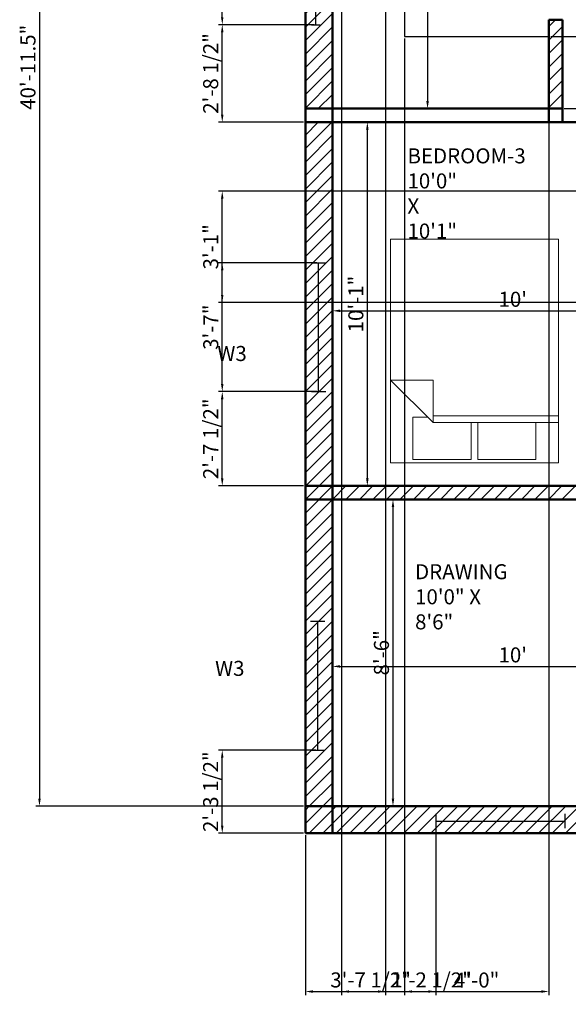
# Model space of a CAD drawing. Units: millimetres. Extents: x 2600 to 3013, y 1440 to 2066.
# Tile 1 of 4: x 2600 to 2782, y 1440 to 1768. Entities that reach past the tile are written whole.
import ezdxf

# ---------------------------------------------------------------- set-up
doc = ezdxf.new("R2010")
doc.units = ezdxf.units.MM
for name, color, linetype, lineweight in [('A-AREA-IDEN', 130, 'Continuous', 25), ('A-FLOR-CASE', 8, 'Continuous', 25), ('A-WALL-PATT', 90, 'Continuous', 13), ('dimensions', 50, 'Continuous', 18), ('furniture', 160, 'Continuous', 18), ('text', 130, 'Continuous', 18), ('walls', 90, 'Continuous', 50), ('windows', 30, 'Continuous', 25)]:
    doc.layers.add(name, color=color, linetype=linetype, lineweight=lineweight)
doc.styles.get("Standard").update_dxf_attribs({"font": 'arial.ttf'})
doc.dimstyles.new('ISO-25', dxfattribs={"dimtxt": 5, "dimasz": 2.5, "dimexe": 1.25, "dimexo": 0.625, "dimtad": 1, "dimdec": 1, "dimlunit": 3, "dimtxsty": 'Standard', "dimcen": 2.5, "dimadec": 0, "dimazin": 0, "dimtfac": 1, "dimtdec": 1, "dimtmove": 0, "dimatfit": 3, "dimfxl": 1, "dimarcsym": 0})

# ---------------------------------------------------------------- blocks, each defined once
blk = doc.blocks.new('*U4')
for p, q in [((0, 4), (0, 0)), ((0, 2), (36, 2)), ((36, 4), (36, 0))]:
    blk.add_line(p, q)
blk = doc.blocks.new('*U5')
for p, q in [((0, 4), (0, 0)), ((36, 4), (36, 0)), ((0, 2), (36, 2))]:
    blk.add_line(p, q)
blk = doc.blocks.new('Bed - Queen')
for p, q in [((0, -80.00003), (0, 0)), ((0, 0), (59.99999, 0)), ((59.99999, 0), (59.99999, -80.00003)), ((7.99999, -1.2), (28.79998, -1.2)), ((7.99999, -14.4), (7.99999, -1.2)), ((28.79998, -1.2), (28.79998, -14.4)), ((31.19999, -1.2), (51.99999, -1.2)), ((31.19999, -14.4), (31.19999, -1.2)), ((51.99999, -1.2), (51.99999, -16.4)), ((0, -14.4), (44.8, -14.4)), ((44.8, -16.8), (0, -16.8)), ((59.99999, -29.6), (44.8, -14.4)), ((44.8, -14.4), (44.8, -29.6)), ((51.99999, -16.4), (46.79936, -16.4)), ((44.8, -29.6), (59.99999, -29.6)), ((59.99999, -80.00003), (0, -80.00003))]:
    blk.add_line(p, q)
blk = doc.blocks.new('*D14')
at = {"layer": 'Defpoints', "color": 0, "transparency": 16777216}
for p in [(2735.41, 1834.18), (2735.41, 1738.18), (2735.41, 1738.18)]:
    blk.add_point(p, dxfattribs=at)
at = {"layer": 'dimensions', "color": 0, "lineweight": -2, "transparency": 16777216}
for p, q in [((2736.04, 1834.18), (2736.66, 1834.18)), ((2735.41, 1831.68), (2735.41, 1740.68)), ((2736.04, 1738.18), (2736.66, 1738.18))]:
    blk.add_line(p, q, dxfattribs=at)
at = {"layer": 'dimensions', "color": 0, "transparency": 16777216}
for points in [[(2735, 1831.68), (2735.83, 1831.68), (2735.41, 1834.18)], [(2735, 1740.68), (2735.83, 1740.68), (2735.41, 1738.18)]]:
    blk.add_solid(points, dxfattribs=at)
at = {"layer": 'dimensions', "color": 0, "transparency": 16777216, "insert": (2732.24, 1786.18), "char_height": 5, "attachment_point": 5, "rotation": 90}
blk.add_mtext("8'", dxfattribs=at)
blk = doc.blocks.new('*D18')
at = {"layer": 'Defpoints', "color": 0, "transparency": 16777216}
for p in [(2823.76, 1552.66), (2703.76, 1535.62), (2823.76, 1535.62)]:
    blk.add_point(p, dxfattribs=at)
at = {"layer": 'dimensions', "color": 0, "lineweight": -2, "transparency": 16777216}
for p, q in [((2703.76, 1536.24), (2703.76, 1553.91)), ((2706.26, 1552.66), (2821.26, 1552.66)), ((2823.76, 1536.24), (2823.76, 1553.91))]:
    blk.add_line(p, q, dxfattribs=at)
at = {"layer": 'dimensions', "color": 0, "transparency": 16777216}
for points in [[(2706.26, 1553.08), (2706.26, 1552.24), (2703.76, 1552.66)], [(2821.26, 1553.08), (2821.26, 1552.24), (2823.76, 1552.66)]]:
    blk.add_solid(points, dxfattribs=at)
at = {"layer": 'dimensions', "color": 0, "transparency": 16777216, "insert": (2763.76, 1555.84), "char_height": 5, "attachment_point": 5}
blk.add_mtext("10'", dxfattribs=at)
blk = doc.blocks.new('*D19')
at = {"layer": 'Defpoints', "color": 0, "transparency": 16777216}
for p in [(2710.05, 1608.18), (2710.05, 1506.18), (2723.9, 1506.18)]:
    blk.add_point(p, dxfattribs=at)
at = {"layer": 'dimensions', "color": 0, "lineweight": -2, "transparency": 16777216}
for p, q in [((2710.67, 1608.18), (2725.15, 1608.18)), ((2723.9, 1605.68), (2723.9, 1508.68)), ((2710.67, 1506.18), (2725.15, 1506.18))]:
    blk.add_line(p, q, dxfattribs=at)
at = {"layer": 'dimensions', "color": 0, "transparency": 16777216}
for points in [[(2723.49, 1605.68), (2724.32, 1605.68), (2723.9, 1608.18)], [(2723.49, 1508.68), (2724.32, 1508.68), (2723.9, 1506.18)]]:
    blk.add_solid(points, dxfattribs=at)
at = {"layer": 'dimensions', "color": 0, "transparency": 16777216, "insert": (2720.72, 1557.18), "char_height": 5, "attachment_point": 5, "rotation": 90}
blk.add_mtext('8\'-6"', dxfattribs=at)
blk = doc.blocks.new('*D22')
at = {"layer": 'Defpoints', "color": 0, "transparency": 16777216}
for p in [(2703.76, 1677.24), (2823.76, 1677.24), (2823.76, 1670.93)]:
    blk.add_point(p, dxfattribs=at)
at = {"layer": 'dimensions', "color": 0, "lineweight": -2, "transparency": 16777216}
for p, q in [((2703.76, 1676.61), (2703.76, 1669.68)), ((2823.76, 1676.61), (2823.76, 1669.68)), ((2706.26, 1670.93), (2821.26, 1670.93))]:
    blk.add_line(p, q, dxfattribs=at)
at = {"layer": 'dimensions', "color": 0, "transparency": 16777216}
for points in [[(2706.26, 1671.35), (2706.26, 1670.51), (2703.76, 1670.93)], [(2821.26, 1671.35), (2821.26, 1670.51), (2823.76, 1670.93)]]:
    blk.add_solid(points, dxfattribs=at)
at = {"layer": 'dimensions', "color": 0, "transparency": 16777216, "insert": (2763.76, 1674.11), "char_height": 5, "attachment_point": 5}
blk.add_mtext("10'", dxfattribs=at)
blk = doc.blocks.new('*D23')
at = {"layer": 'Defpoints', "color": 0, "transparency": 16777216}
for p in [(2710.27, 1733.68), (2715.38, 1733.68), (2710.27, 1612.68)]:
    blk.add_point(p, dxfattribs=at)
at = {"layer": 'dimensions', "color": 0, "lineweight": -2, "transparency": 16777216}
for p, q in [((2710.89, 1733.68), (2716.63, 1733.68)), ((2715.38, 1615.18), (2715.38, 1731.18)), ((2710.89, 1612.68), (2716.63, 1612.68))]:
    blk.add_line(p, q, dxfattribs=at)
at = {"layer": 'dimensions', "color": 0, "transparency": 16777216}
for points in [[(2714.96, 1731.18), (2715.8, 1731.18), (2715.38, 1733.68)], [(2714.96, 1615.18), (2715.8, 1615.18), (2715.38, 1612.68)]]:
    blk.add_solid(points, dxfattribs=at)
at = {"layer": 'dimensions', "color": 0, "transparency": 16777216, "insert": (2712.2, 1673.18), "char_height": 5, "attachment_point": 5, "rotation": 90}
blk.add_mtext('10\'-1"', dxfattribs=at)
blk = doc.blocks.new('*D28')
at = {"layer": 'Defpoints', "color": 0, "transparency": 16777216}
for p in [(2694.76, 1997.68), (2606.3, 1506.18), (2694.76, 1506.18)]:
    blk.add_point(p, dxfattribs=at)
at = {"layer": 'dimensions', "color": 0, "lineweight": -2, "transparency": 16777216}
for p, q in [((2694.13, 1997.68), (2605.05, 1997.68)), ((2606.3, 1995.18), (2606.3, 1508.68)), ((2694.13, 1506.18), (2605.05, 1506.18))]:
    blk.add_line(p, q, dxfattribs=at)
at = {"layer": 'dimensions', "color": 0, "transparency": 16777216}
for points in [[(2605.88, 1995.18), (2606.72, 1995.18), (2606.3, 1997.68)], [(2605.88, 1508.68), (2606.72, 1508.68), (2606.3, 1506.18)]]:
    blk.add_solid(points, dxfattribs=at)
at = {"layer": 'dimensions', "color": 0, "transparency": 16777216, "insert": (2603.12, 1751.93), "char_height": 5, "attachment_point": 5, "rotation": 90}
blk.add_mtext('40\'-11.5"', dxfattribs=at)
blk = doc.blocks.new('*D41')
at = {"layer": 'Defpoints', "color": 0, "transparency": 16777216}
for p in [(2667.11, 1792.07), (2698.28, 1792.07), (2698.28, 1766.09)]:
    blk.add_point(p, dxfattribs=at)
at = {"layer": 'dimensions', "color": 0, "lineweight": -2, "transparency": 16777216}
for p, q in [((2697.66, 1792.07), (2665.86, 1792.07)), ((2667.11, 1768.59), (2667.11, 1789.57)), ((2697.66, 1766.09), (2665.86, 1766.09))]:
    blk.add_line(p, q, dxfattribs=at)
at = {"layer": 'dimensions', "color": 0, "transparency": 16777216}
for points in [[(2666.69, 1789.57), (2667.52, 1789.57), (2667.11, 1792.07)], [(2666.69, 1768.59), (2667.52, 1768.59), (2667.11, 1766.09)]]:
    blk.add_solid(points, dxfattribs=at)
at = {"layer": 'dimensions', "color": 0, "transparency": 16777216, "insert": (2663.97, 1779.08), "char_height": 5, "attachment_point": 5, "rotation": 90}
blk.add_mtext('2\'-2"', dxfattribs=at)
blk = doc.blocks.new('*D42')
at = {"layer": 'Defpoints', "color": 0, "transparency": 16777216}
for p in [(2667.11, 1686.94), (2699.16, 1686.94), (2699.16, 1644.04)]:
    blk.add_point(p, dxfattribs=at)
at = {"layer": 'dimensions', "color": 0, "lineweight": -2, "transparency": 16777216}
for p, q in [((2698.54, 1686.94), (2665.86, 1686.94)), ((2667.11, 1646.54), (2667.11, 1684.44)), ((2698.54, 1644.04), (2665.86, 1644.04))]:
    blk.add_line(p, q, dxfattribs=at)
at = {"layer": 'dimensions', "color": 0, "transparency": 16777216}
for points in [[(2666.69, 1684.44), (2667.52, 1684.44), (2667.11, 1686.94)], [(2666.69, 1646.54), (2667.52, 1646.54), (2667.11, 1644.04)]]:
    blk.add_solid(points, dxfattribs=at)
at = {"layer": 'dimensions', "color": 0, "transparency": 16777216, "insert": (2663.93, 1665.49), "char_height": 5, "attachment_point": 5, "rotation": 90}
blk.add_mtext('3\'-7"', dxfattribs=at)
blk = doc.blocks.new('*D45')
at = {"layer": 'Defpoints', "color": 0, "transparency": 16777216}
for p in [(2727.76, 1762.18), (2775.76, 1762.18), (2775.76, 1444.53)]:
    blk.add_point(p, dxfattribs=at)
at = {"layer": 'dimensions', "color": 0, "lineweight": -2, "transparency": 16777216}
for p, q in [((2727.76, 1761.55), (2727.76, 1443.28)), ((2775.76, 1761.55), (2775.76, 1443.28)), ((2730.26, 1444.53), (2773.26, 1444.53))]:
    blk.add_line(p, q, dxfattribs=at)
at = {"layer": 'dimensions', "color": 0, "transparency": 16777216}
for points in [[(2730.26, 1444.94), (2730.26, 1444.11), (2727.76, 1444.53)], [(2773.26, 1444.94), (2773.26, 1444.11), (2775.76, 1444.53)]]:
    blk.add_solid(points, dxfattribs=at)
at = {"layer": 'dimensions', "color": 0, "transparency": 16777216, "insert": (2751.76, 1447.71), "char_height": 5, "attachment_point": 5}
blk.add_mtext('4\'-0"', dxfattribs=at)
blk = doc.blocks.new('*D46')
at = {"layer": 'Defpoints', "color": 0, "transparency": 16777216}
for p in [(2775.76, 1762.18), (3008.91, 1762.18), (2780.26, 1738.18)]:
    blk.add_point(p, dxfattribs=at)
at = {"layer": 'dimensions', "color": 0, "lineweight": -2, "transparency": 16777216}
for p, q in [((2776.38, 1762.18), (3010.16, 1762.18)), ((3008.91, 1740.68), (3008.91, 1759.68)), ((2780.88, 1738.18), (3010.16, 1738.18))]:
    blk.add_line(p, q, dxfattribs=at)
at = {"layer": 'dimensions', "color": 0, "transparency": 16777216}
for points in [[(3008.49, 1759.68), (3009.32, 1759.68), (3008.91, 1762.18)], [(3008.49, 1740.68), (3009.32, 1740.68), (3008.91, 1738.18)]]:
    blk.add_solid(points, dxfattribs=at)
at = {"layer": 'dimensions', "color": 0, "transparency": 16777216, "insert": (3005.73, 1750.18), "char_height": 5, "attachment_point": 5, "rotation": 90}
blk.add_mtext('2\'-0"', dxfattribs=at)
blk = doc.blocks.new('*D48')
at = {"layer": 'Defpoints', "color": 0, "transparency": 16777216}
for p in [(2706.82, 1786.43), (2721.39, 1786.43), (2721.39, 1444.53)]:
    blk.add_point(p, dxfattribs=at)
at = {"layer": 'dimensions', "color": 0, "lineweight": -2, "transparency": 16777216}
for p, q in [((2706.82, 1785.8), (2706.82, 1443.28)), ((2721.39, 1785.8), (2721.39, 1443.28)), ((2709.32, 1444.53), (2718.89, 1444.53)), ((2721.39, 1444.53), (2749.61, 1444.53))]:
    blk.add_line(p, q, dxfattribs=at)
at = {"layer": 'dimensions', "color": 0, "transparency": 16777216}
for points in [[(2709.32, 1444.94), (2709.32, 1444.11), (2706.82, 1444.53)], [(2718.89, 1444.94), (2718.89, 1444.11), (2721.39, 1444.53)]]:
    blk.add_solid(points, dxfattribs=at)
at = {"layer": 'dimensions', "color": 0, "transparency": 16777216, "insert": (2736.75, 1447.74), "char_height": 5, "attachment_point": 5}
blk.add_mtext('1\'-2 1/2"', dxfattribs=at)
blk = doc.blocks.new('*D52')
at = {"layer": 'Defpoints', "color": 0, "transparency": 16777216}
for p in [(2667.11, 1766.09), (2698.28, 1766.09), (2694.76, 1733.68)]:
    blk.add_point(p, dxfattribs=at)
at = {"layer": 'dimensions', "color": 0, "lineweight": -2, "transparency": 16777216}
for p, q in [((2697.66, 1766.09), (2665.86, 1766.09)), ((2667.11, 1736.18), (2667.11, 1763.59)), ((2694.13, 1733.68), (2665.86, 1733.68))]:
    blk.add_line(p, q, dxfattribs=at)
at = {"layer": 'dimensions', "color": 0, "transparency": 16777216}
for points in [[(2666.69, 1763.59), (2667.52, 1763.59), (2667.11, 1766.09)], [(2666.69, 1736.18), (2667.52, 1736.18), (2667.11, 1733.68)]]:
    blk.add_solid(points, dxfattribs=at)
at = {"layer": 'dimensions', "color": 0, "transparency": 16777216, "insert": (2663.9, 1749.88), "char_height": 5, "attachment_point": 5, "rotation": 90}
blk.add_mtext('2\'-8 1/2"', dxfattribs=at)
blk = doc.blocks.new('*D54')
at = {"layer": 'Defpoints', "color": 0, "transparency": 16777216}
for p in [(2667.11, 1524.81), (2698.9, 1524.81), (2694.76, 1497.18)]:
    blk.add_point(p, dxfattribs=at)
at = {"layer": 'dimensions', "color": 0, "lineweight": -2, "transparency": 16777216}
for p, q in [((2698.27, 1524.81), (2665.86, 1524.81)), ((2667.11, 1499.68), (2667.11, 1522.31)), ((2694.13, 1497.18), (2665.86, 1497.18))]:
    blk.add_line(p, q, dxfattribs=at)
at = {"layer": 'dimensions', "color": 0, "transparency": 16777216}
for points in [[(2666.69, 1522.31), (2667.52, 1522.31), (2667.11, 1524.81)], [(2666.69, 1499.68), (2667.52, 1499.68), (2667.11, 1497.18)]]:
    blk.add_solid(points, dxfattribs=at)
at = {"layer": 'dimensions', "color": 0, "transparency": 16777216, "insert": (2663.89, 1511), "char_height": 5, "attachment_point": 5, "rotation": 90}
blk.add_mtext('2\'-3 1/2"', dxfattribs=at)
blk = doc.blocks.new('*D56')
at = {"layer": 'Defpoints', "color": 0, "transparency": 16777216}
for p in [(2667.11, 1644.04), (2699.16, 1644.04), (2694.76, 1612.68)]:
    blk.add_point(p, dxfattribs=at)
at = {"layer": 'dimensions', "color": 0, "lineweight": -2, "transparency": 16777216}
for p, q in [((2698.54, 1644.04), (2665.86, 1644.04)), ((2667.11, 1615.18), (2667.11, 1641.54)), ((2694.13, 1612.68), (2665.86, 1612.68))]:
    blk.add_line(p, q, dxfattribs=at)
at = {"layer": 'dimensions', "color": 0, "transparency": 16777216}
for points in [[(2666.69, 1641.54), (2667.52, 1641.54), (2667.11, 1644.04)], [(2666.69, 1615.18), (2667.52, 1615.18), (2667.11, 1612.68)]]:
    blk.add_solid(points, dxfattribs=at)
at = {"layer": 'dimensions', "color": 0, "transparency": 16777216, "insert": (2663.9, 1628.36), "char_height": 5, "attachment_point": 5, "rotation": 90}
blk.add_mtext('2\'-7 1/2"', dxfattribs=at)
blk = doc.blocks.new('*D58')
at = {"layer": 'Defpoints', "color": 0, "transparency": 16777216}
for p in [(2667.11, 1710.7), (2976.63, 1710.7), (2977.46, 1673.74)]:
    blk.add_point(p, dxfattribs=at)
at = {"layer": 'dimensions', "color": 0, "lineweight": -2, "transparency": 16777216}
for p, q in [((2976, 1710.7), (2665.86, 1710.7)), ((2667.11, 1676.24), (2667.11, 1708.2)), ((2976.83, 1673.74), (2665.86, 1673.74))]:
    blk.add_line(p, q, dxfattribs=at)
at = {"layer": 'dimensions', "color": 0, "transparency": 16777216}
for points in [[(2666.69, 1708.2), (2667.52, 1708.2), (2667.11, 1710.7)], [(2666.69, 1676.24), (2667.52, 1676.24), (2667.11, 1673.74)]]:
    blk.add_solid(points, dxfattribs=at)
at = {"layer": 'dimensions', "color": 0, "transparency": 16777216, "insert": (2663.93, 1692.22), "char_height": 5, "attachment_point": 5, "rotation": 90}
blk.add_mtext('3\'-1"', dxfattribs=at)
blk = doc.blocks.new('*D59')
at = {"layer": 'Defpoints', "color": 0, "transparency": 16777216}
for p in [(2738.19, 1501.22), (2694.76, 1497.18), (2738.19, 1444.53)]:
    blk.add_point(p, dxfattribs=at)
at = {"layer": 'dimensions', "color": 0, "lineweight": -2, "transparency": 16777216}
for p, q in [((2738.19, 1500.59), (2738.19, 1443.28)), ((2694.76, 1496.55), (2694.76, 1443.28)), ((2697.26, 1444.53), (2735.69, 1444.53))]:
    blk.add_line(p, q, dxfattribs=at)
at = {"layer": 'dimensions', "color": 0, "transparency": 16777216}
for points in [[(2697.26, 1444.94), (2697.26, 1444.11), (2694.76, 1444.53)], [(2735.69, 1444.94), (2735.69, 1444.11), (2738.19, 1444.53)]]:
    blk.add_solid(points, dxfattribs=at)
at = {"layer": 'dimensions', "color": 0, "transparency": 16777216, "insert": (2716.47, 1447.74), "char_height": 5, "attachment_point": 5}
blk.add_mtext('3\'-7 1/2"', dxfattribs=at)

msp = doc.modelspace()

# ---------------------------------------------------------------- hatches: boundary and pattern name
at = {"layer": 'A-WALL-PATT'}
h = msp.add_hatch(dxfattribs=at)
h.set_pattern_fill('ANSI31', color=256)
h.paths.add_polyline_path([(2972.26, 1997.68), (2828.26, 1997.68), (2828.26, 1988.68), (2972.26, 1988.68)])
h.paths.add_polyline_path([(2823.76, 1997.68), (2703.76, 1997.68), (2703.76, 1988.68), (2823.76, 1988.68)])
h.paths.add_polyline_path([(2828.26, 1997.68), (2823.76, 1997.68), (2823.76, 1988.68), (2828.26, 1988.68)])
h.paths.add_polyline_path([(2703.76, 1997.68), (2694.76, 1997.68), (2694.76, 1988.68), (2703.76, 1988.68)])
h.paths.add_polyline_path([(2703.76, 1988.68), (2694.76, 1988.68), (2694.76, 1958.65), (2698.77, 1958.65), (2698.77, 1886.48), (2694.76, 1886.48), (2694.76, 1838.68), (2703.76, 1838.68)])
h.paths.add_polyline_path([(2703.76, 1733.68), (2694.76, 1733.68), (2694.76, 1612.68), (2703.76, 1612.68)])
h.paths.add_polyline_path([(2703.76, 1608.18), (2694.76, 1608.18), (2694.76, 1506.18), (2703.76, 1506.18)])
h.paths.add_polyline_path([(2703.76, 1612.68), (2694.76, 1612.68), (2694.76, 1608.18), (2703.76, 1608.18)])
h.paths.add_polyline_path([(2823.76, 1612.68), (2703.76, 1612.68), (2703.76, 1608.18), (2823.76, 1608.18)])
h.paths.add_polyline_path([(2972.26, 1611.68), (2869.05, 1611.68, -0.005663), (2869.06, 1610.86), (2869.06, 1607.18), (2972.26, 1607.18)])
h.paths.add_polyline_path([(2981.26, 1607.18), (2972.26, 1607.18), (2972.26, 1506.18), (2981.26, 1506.18)])
h.paths.add_polyline_path([(2981.26, 1611.68), (2972.26, 1611.68), (2972.26, 1607.18), (2981.26, 1607.18)])
h.paths.add_polyline_path([(2828.26, 1569.75), (2824.68, 1569.8, -0.006355), (2823.76, 1569.82), (2823.76, 1506.18), (2828.26, 1506.18)])
h.paths.add_polyline_path([(2828.26, 1733.68), (2823.76, 1733.68), (2823.76, 1612.68), (2828.26, 1612.68)])
h.paths.add_polyline_path([(2981.26, 1783.68), (2972.26, 1783.68), (2972.26, 1611.68), (2981.26, 1611.68)])
h.paths.add_polyline_path([(2972.26, 1838.68), (2883.26, 1838.68), (2883.26, 1834.18), (2972.26, 1834.18)])
h.paths.add_polyline_path([(2981.26, 1838.68), (2972.26, 1838.68), (2972.26, 1834.18), (2981.26, 1834.18)])
h.paths.add_polyline_path([(2981.26, 1834.18), (2972.26, 1834.18), (2972.26, 1788.18), (2981.26, 1788.18)])
h.paths.add_polyline_path([(2981.26, 1988.68), (2972.26, 1988.68), (2972.26, 1952.13), (2976.27, 1952.13), (2976.27, 1879.95), (2972.26, 1879.95), (2972.26, 1838.68), (2981.26, 1838.68)])
h.paths.add_polyline_path([(2828.26, 1988.68), (2823.76, 1988.68), (2823.76, 1838.68), (2828.26, 1838.68)])
h.paths.add_polyline_path([(2780.26, 1834.18), (2775.76, 1834.18), (2775.76, 1799.5), (2780.26, 1799.5)])
h.paths.add_polyline_path([(2775.76, 1838.68), (2703.76, 1838.68), (2703.76, 1834.18), (2775.76, 1834.18)])
h.paths.add_polyline_path([(2780.26, 1838.68), (2775.76, 1838.68), (2775.76, 1834.18), (2780.26, 1834.18)])
h.paths.add_polyline_path([(2828.26, 1838.68), (2823.76, 1838.68), (2823.76, 1834.18), (2828.26, 1834.18)])
h.paths.add_polyline_path([(2883.26, 1838.68), (2878.76, 1838.68), (2878.76, 1834.18), (2883.26, 1834.18)])
h.paths.add_polyline_path([(2886.68, 1812.39), (2892.39, 1812.39), (2892.39, 1817.54), (2886.68, 1817.54)], flags=9)
h = msp.add_hatch(dxfattribs=at)
h.set_pattern_fill('ANSI31', color=256)
h.paths.add_polyline_path([(2703.76, 1834.18), (2694.76, 1834.18), (2694.76, 1738.18), (2703.76, 1738.18)])
h.paths.add_polyline_path([(2780.26, 1767.75), (2775.76, 1767.75), (2775.76, 1738.18), (2780.26, 1738.18)])
h.paths.add_polyline_path([(2972.26, 1506.18), (2868.8, 1506.18, -0.033203), (2869.12, 1501.37), (2869.12, 1497.18), (2972.26, 1497.18)])
h.paths.add_polyline_path([(2981.26, 1506.18), (2972.26, 1506.18), (2972.26, 1497.18), (2981.26, 1497.18)])
h.paths.add_polyline_path([(2823.76, 1506.18), (2703.76, 1506.18), (2703.76, 1497.18), (2823.76, 1497.18)])
h.paths.add_polyline_path([(2828.26, 1506.18), (2823.76, 1506.18), (2823.76, 1497.18), (2828.26, 1497.18)])
h.paths.add_polyline_path([(2832.8, 1506.18), (2828.26, 1506.18), (2828.26, 1497.18), (2832.8, 1497.18), (2832.8, 1501.37)])
h.paths.add_polyline_path([(2703.76, 1506.18), (2694.76, 1506.18), (2694.76, 1497.18), (2703.76, 1497.18)])
h.paths.add_polyline_path([(2981.26, 1997.68), (2972.26, 1997.68), (2972.26, 1988.68), (2981.26, 1988.68)])

# ---------------------------------------------------------------- linework, layer by layer
at = {"layer": 'A-FLOR-CASE'}
for p, q in [((2727.76, 1825.08), (2727.76, 1762.18)), ((2727.76, 1762.18), (2775.76, 1762.18))]:
    msp.add_line(p, q, dxfattribs=at)
at = {"layer": 'walls'}
for p, q in [((2694.76, 1997.68), (2694.76, 1497.18)), ((2703.76, 1997.68), (2703.76, 1497.18)), ((2775.76, 1767.75), (2780.26, 1767.75)), ((2775.76, 1767.75), (2775.76, 1733.68)), ((2775.76, 1767.75), (2775.76, 1733.68)), ((2780.26, 1767.75), (2780.26, 1733.68)), ((2780.26, 1767.75), (2780.26, 1733.68)), ((2694.76, 1738.18), (2780.26, 1738.18)), ((2694.76, 1733.68), (2828.26, 1733.68)), ((2694.76, 1612.68), (2828.26, 1612.68)), ((2694.76, 1608.18), (2828.26, 1608.18)), ((2694.76, 1506.18), (2834.39, 1506.18)), ((2694.76, 1497.18), (2981.26, 1497.18))]:
    msp.add_line(p, q, dxfattribs=at)

# ---------------------------------------------------------------- block references
at = {"layer": 'furniture', "xscale": 0.9302566542625909, "yscale": 0.9302566542625909, "zscale": 0.9302566542625909, "rotation": 179.9999999999988}
msp.add_blockref('Bed - Queen', (2778.93, 1620.34), dxfattribs=at)
at = {"layer": 'windows', "rotation": 90}
for name, p, xscale, yscale, zscale in [('*U4', (2699.73, 1766.09), 0.7216899638288952, 0.7216899638288952, 0.7216899638288952), ('*U5', (2701.55, 1644.04), 1.191580422458004, 1.191580422458004, 1.191580422458004), ('*U5', (2701.28, 1524.81), 1.191580422458004, 1.191580422458004, 1.191580422458004)]:
    msp.add_blockref(name, p, dxfattribs=dict(at, xscale=xscale, yscale=yscale, zscale=zscale))
at = {"layer": 'windows', "xscale": 1.191580422458004, "yscale": 1.191580422458004, "zscale": 1.191580422458004}
msp.add_blockref('*U5', (2738.19, 1498.83), dxfattribs=at)

# ---------------------------------------------------------------- texts
at = {"layer": 'A-AREA-IDEN', "char_height": 5, "attachment_point": 1}
for s, width, insert in [('BEDROOM-3\\P10\'0" X 10\'1"', 20.1528, (2728.73, 1724.96)), ('DRAWING\\P10\'0" X 8\'6"', 22.8851, (2731.26, 1586.65))]:
    msp.add_mtext_dynamic_manual_height_columns(s, width=width, gutter_width=12.5, heights=[0], dxfattribs=dict(at, insert=insert))
at = {"layer": 'text', "char_height": 5, "attachment_point": 1}
for width, insert in [(22.288, (2665.49, 1659.23)), (12.3846, (2664.73, 1554.51))]:
    msp.add_mtext_dynamic_manual_height_columns('W3', width=width, gutter_width=12.5, heights=[0], dxfattribs=dict(at, insert=insert))

# ---------------------------------------------------------------- dimensions: what is measured, and where the dimension line sits
at = {"layer": 'dimensions'}
for base, p1, p2, override, picture, middle in [((2606.3, 1506.18), (2694.76, 1997.68), (2694.76, 1506.18), {"dimclrd": 0, "dimclre": 0, "dimclrt": 0}, '*D28', (2603.12, 1751.93)), ((2735.41, 1738.18), (2735.41, 1834.18), (2735.41, 1738.18), {"dimclrd": 0, "dimclre": 0, "dimclrt": 0}, '*D14', (2732.24, 1786.18)), ((2667.11, 1792.07), (2698.28, 1766.09), (2698.28, 1792.07), {"dimdec": 1, "dimlfac": 1, "dimrnd": 0, "dimzin": 1, "dimdsep": 46, "dimlunit": 4, "dimfrac": 2}, '*D41', (2663.97, 1779.08)), ((2667.11, 1766.09), (2694.76, 1733.68), (2698.28, 1766.09), {"dimdec": 1, "dimlfac": 1, "dimrnd": 0, "dimzin": 1, "dimdsep": 46, "dimlunit": 4, "dimfrac": 2}, '*D52', (2663.9, 1749.88)), ((3008.91, 1762.18), (2780.26, 1738.18), (2775.76, 1762.18), {"dimdec": 1, "dimlfac": 1, "dimrnd": 0, "dimzin": 1, "dimdsep": 46, "dimlunit": 4, "dimfrac": 2}, '*D46', (3005.73, 1750.18)), ((2715.38, 1733.68), (2710.27, 1612.68), (2710.27, 1733.68), {"dimclrd": 0, "dimclre": 0, "dimclrt": 0}, '*D23', (2712.2, 1673.18)), ((2667.11, 1710.7), (2977.46, 1673.74), (2976.63, 1710.7), {"dimdec": 1, "dimlfac": 1, "dimrnd": 0, "dimzin": 1, "dimdsep": 46, "dimlunit": 4, "dimfrac": 2}, '*D58', (2663.93, 1692.22)), ((2667.11, 1686.94), (2699.16, 1644.04), (2699.16, 1686.94), {"dimdec": 1, "dimlfac": 1, "dimrnd": 0, "dimzin": 1, "dimdsep": 46, "dimlunit": 4, "dimfrac": 2}, '*D42', (2663.93, 1665.49)), ((2667.11, 1644.04), (2694.76, 1612.68), (2699.16, 1644.04), {"dimdec": 1, "dimlfac": 1, "dimrnd": 0, "dimzin": 1, "dimdsep": 46, "dimlunit": 4, "dimfrac": 2}, '*D56', (2663.9, 1628.36)), ((2723.9, 1506.18), (2710.05, 1608.18), (2710.05, 1506.18), {"dimclrd": 0, "dimclre": 0, "dimclrt": 0}, '*D19', (2720.72, 1557.18)), ((2667.11, 1524.81), (2694.76, 1497.18), (2698.9, 1524.81), {"dimdec": 1, "dimlfac": 1, "dimrnd": 0, "dimzin": 1, "dimdsep": 46, "dimlunit": 4, "dimfrac": 2}, '*D54', (2663.89, 1511))]:
    dim = msp.add_linear_dim(base=base, p1=p1, p2=p2, angle=90, dimstyle='ISO-25', override=override, dxfattribs=at)
    dim.commit()
    dim.dimension.update_dxf_attribs({"geometry": picture, "text_midpoint": middle})
for base, p1, p2, override, picture, middle in [((2721.39, 1444.53), (2706.82, 1786.43), (2721.39, 1786.43), {"dimdec": 1, "dimlfac": 1, "dimrnd": 0, "dimzin": 1, "dimdsep": 46, "dimlunit": 4, "dimfrac": 2}, '*D48', (2736.75, 1447.74)), ((2775.76, 1444.53), (2727.76, 1762.18), (2775.76, 1762.18), {"dimdec": 1, "dimlfac": 1, "dimrnd": 0, "dimzin": 1, "dimdsep": 46, "dimlunit": 4, "dimfrac": 2}, '*D45', (2751.76, 1447.71)), ((2823.76, 1670.93), (2703.76, 1677.24), (2823.76, 1677.24), {"dimclrd": 0, "dimclre": 0, "dimclrt": 0}, '*D22', (2763.76, 1674.11)), ((2823.76, 1552.66), (2703.76, 1535.62), (2823.76, 1535.62), {"dimclrd": 0, "dimclre": 0, "dimclrt": 0}, '*D18', (2763.76, 1555.84)), ((2738.19, 1444.53), (2694.76, 1497.18), (2738.19, 1501.22), {"dimdec": 1, "dimlfac": 1, "dimrnd": 0, "dimzin": 1, "dimdsep": 46, "dimlunit": 4, "dimfrac": 2}, '*D59', (2716.47, 1447.74))]:
    dim = msp.add_linear_dim(base=base, p1=p1, p2=p2, dimstyle='ISO-25', override=override, dxfattribs=at)
    dim.commit()
    dim.dimension.update_dxf_attribs({"geometry": picture, "text_midpoint": middle})

doc.saveas('drawing.dxf')
